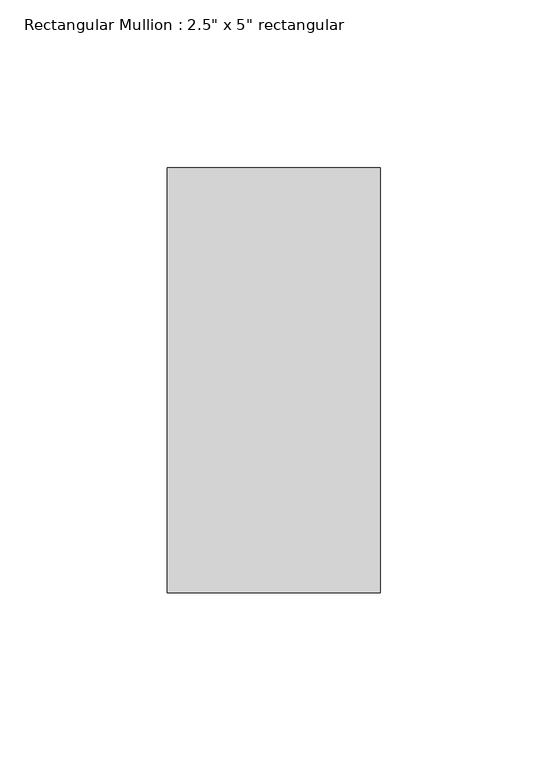
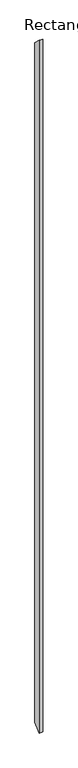
"""IFC4 building model written with IfcOpenShell, lengths in millimetres: member geometry."""

from ifc_helpers import new_model, si_unit, frame, origin, place, context, project, spatial, polyline, outline, extrude, source, transform, mapped, element, save


def member_d818a040(model_context):
    return source(origin(), model_context, "Body", "SweptSolid", [
        extrude(outline(polyline([(-63.5, 63.5), (63.5, -63.5), (63.5, -12758.7552746), (-63.5, -12885.7552746), (-63.5, 63.5)])), frame((-63.5, 0.0, 0.0), z_axis=(1.0, 0.0, 0.0), x_axis=(0.0, 1.0, 0.0)), (0.0, 0.0, 1.0), 63.5),
    ])


if __name__ == "__main__":
    model = new_model("IFC4")
    model_context = context("Model", 3, world=origin())
    ifc_project = project(units=[si_unit("LENGTHUNIT", "METRE", prefix="MILLI")], contexts=[model_context])
    site = spatial("IfcSite", under=ifc_project)
    building = spatial("IfcBuilding", under=site)
    placement = place(None, origin())
    member_shape = member_d818a040(model_context)
    element("IfcMember", 1, ObjectType="Rectangular Mullion : 2.5\" x 5\" rectangular", at=placement, inside=building, context=model_context, shape_type="MappedRepresentation", body=[
        mapped(member_shape, transform((0.0, 0.0, 0.0), x_axis=(1.0, 0.0, 0.0), y_axis=(0.0, 1.0, 0.0), z_axis=(0.0, 0.0, 1.0))),
    ])
    save(model, "model.ifc")

# Revit data of these elements
# Type "Rectangular Mullion : 2.5\" x 5\" rectangular"
#   built-in parameter 1007304 = 0.416667 (stored number, unit not read)
#   built-in parameter 1007301 = 0.104167 (stored number, unit not read)
#   built-in parameter 1007300 = 0.104167 (stored number, unit not read)
# Element 1 (IfcMember, "Rectangular Mullion : 2.5\" x 5\" rectangular")
#   Materials on its faces: "Aluminum"
# Materials
#   "Aluminum": class "Metal", colour RGB 247 247 247, transparency 0, Description = "Aluminum 6061", Cost = 0
